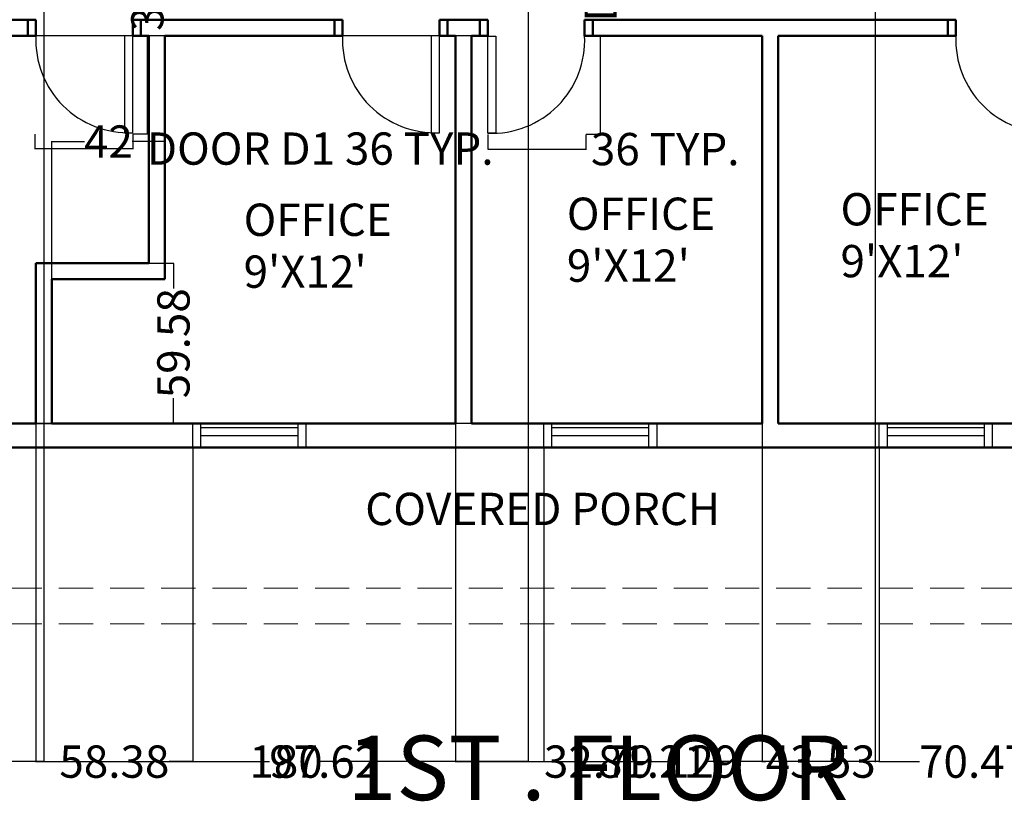
# Model space of a CAD drawing. Units: inches. Extents: x 128 to 1267, y -109 to 1208.
# Tile 2 of 8: x 418 to 784, y -97 to 194. Entities that reach past the tile are written whole.
import ezdxf

# ---------------------------------------------------------------- set-up
doc = ezdxf.new("R2010")
doc.units = ezdxf.units.IN
doc.header["$MEASUREMENT"] = 0
doc.linetypes.add('DASHED', pattern=[19.05, 12.7, -6.35])
for name, color, linetype, lineweight in [('A-ANNO-DIMS', 2, 'Continuous', 18), ('A-ANNO-TEXT', 7, 'Continuous', 35), ('A-AREA-IDEN', 3, 'Continuous', 25), ('A-DOOR', 4, 'Continuous', 25), ('A-GLAZ', 3, 'Continuous', 25), ('A-ROOF-OVHD', 9, 'DASHED', 18), ('A-WALL', 7, 'Continuous', 50)]:
    doc.layers.add(name, color=color, linetype=linetype, lineweight=lineweight)
doc.styles.get("Standard").update_dxf_attribs({"font": 'arial.ttf'})
doc.dimstyles.get("Standard").update_dxf_attribs({"dimtxt": 12, "dimasz": 0.18, "dimexe": 0.18, "dimexo": 0.0625, "dimgap": 0.09, "dimtad": 0, "dimdec": 1, "dimzin": 0, "dimdsep": 46, "dimlunit": 3, "dimtxsty": 'Standard', "dimcen": 0.09, "dimadec": 0, "dimazin": 0, "dimtfac": 1, "dimtdec": 1, "dimtofl": 0, "dimtmove": 0, "dimatfit": 3, "dimfxl": 1, "dimtolj": 1, "dimtzin": 0, "dimarcsym": 0})

# ---------------------------------------------------------------- blocks, each defined once
blk = doc.blocks.new('DOOR-900')
blk.add_lwpolyline([(460.06, 187.64), (457.06, 187.64), (457.06, 151.64), (460.06, 151.64)], close=True)
blk.add_arc((458.56, 186.14), 34.53, 177.5104, 272.4896)
blk = doc.blocks.new('DOOR-875')
blk.add_lwpolyline([(592.06, 187.47), (595.06, 187.47), (595.06, 151.47), (592.06, 151.47)], close=True)
blk.add_arc((593.56, 185.98), 34.54, 267.511, 2.7608)
blk = doc.blocks.new('WIN-900')
for p, q in [((1102.06, 345.56), (1111.06, 345.56)), ((1102.06, 342.56), (1111.06, 342.56)), ((1103.56, 306.56), (1103.56, 342.56)), ((1106.56, 306.56), (1106.56, 342.56)), ((1111.06, 306.56), (1102.06, 306.56)), ((1111.06, 303.56), (1102.06, 303.56))]:
    blk.add_line(p, q)
blk = doc.blocks.new('*D10')
at = {"layer": 'A-ANNO-DIMS', "color": 0, "lineweight": -2, "transparency": 16777216}
for p, q in [((423.64, 151.16), (423.64, 145.58)), ((460.06, 151.16), (460.06, 145.58)), ((423.82, 145.76), (459.88, 145.76)), ((460.06, 145.76), (460.24, 145.76))]:
    blk.add_line(p, q, dxfattribs=at)
at = {"layer": 'A-ANNO-DIMS', "color": 0, "transparency": 16777216}
for points in [[(423.82, 145.79), (423.82, 145.73), (423.64, 145.76)], [(459.88, 145.79), (459.88, 145.73), (460.06, 145.76)]]:
    blk.add_solid(points, dxfattribs=at)
at = {"layer": 'Defpoints', "color": 0, "transparency": 16777216}
for p in [(423.64, 151.22), (460.06, 151.22), (460.06, 145.76)]:
    blk.add_point(p, dxfattribs=at)
at = {"layer": 'A-ANNO-DIMS', "color": 0, "transparency": 16777216, "insert": (529.75, 145.76), "char_height": 12, "attachment_point": 5}
blk.add_mtext('\\A1;DOOR D1 36 TYP.', dxfattribs=at)
blk = doc.blocks.new('*D11')
at = {"layer": 'A-ANNO-DIMS', "color": 0, "lineweight": -2, "transparency": 16777216}
for p, q in [((460.12, 187.64), (465.7, 187.64)), ((465.52, 187.64), (465.52, 187.82)), ((465.52, 151.4), (465.52, 187.46)), ((460.12, 151.22), (465.7, 151.22))]:
    blk.add_line(p, q, dxfattribs=at)
at = {"layer": 'A-ANNO-DIMS', "color": 0, "transparency": 16777216}
for points in [[(465.49, 187.46), (465.55, 187.46), (465.52, 187.64)], [(465.49, 151.4), (465.55, 151.4), (465.52, 151.22)]]:
    blk.add_solid(points, dxfattribs=at)
at = {"layer": 'Defpoints', "color": 0, "transparency": 16777216}
for p in [(460.06, 187.64), (465.52, 187.64), (460.06, 151.22)]:
    blk.add_point(p, dxfattribs=at)
at = {"layer": 'A-ANNO-DIMS', "color": 0, "transparency": 16777216, "insert": (465.52, 217.11), "char_height": 12, "attachment_point": 5, "rotation": 90}
blk.add_mtext('\\A1;36 TYP.', dxfattribs=at)
blk = doc.blocks.new('*D20')
at = {"layer": 'A-ANNO-DIMS', "color": 0, "lineweight": -2, "transparency": 16777216}
for p, q in [((628.59, 187.64), (634.19, 187.64)), ((634.01, 187.64), (634.01, 187.82)), ((634.01, 151.23), (634.01, 187.46)), ((628.59, 151.05), (634.19, 151.05))]:
    blk.add_line(p, q, dxfattribs=at)
at = {"layer": 'A-ANNO-DIMS', "color": 0, "transparency": 16777216}
for points in [[(633.98, 187.46), (634.04, 187.46), (634.01, 187.64)], [(633.98, 151.23), (634.04, 151.23), (634.01, 151.05)]]:
    blk.add_solid(points, dxfattribs=at)
at = {"layer": 'Defpoints', "color": 0, "transparency": 16777216}
for p in [(628.52, 187.64), (634.01, 187.64), (628.52, 151.05)]:
    blk.add_point(p, dxfattribs=at)
at = {"layer": 'A-ANNO-DIMS', "color": 0, "transparency": 16777216, "insert": (634.01, 257.34), "char_height": 12, "attachment_point": 5, "rotation": 90}
blk.add_mtext('\\A1;DOOR D2 37 TYP.', dxfattribs=at)
blk = doc.blocks.new('*D21')
at = {"layer": 'A-ANNO-DIMS', "color": 0, "lineweight": -2, "transparency": 16777216}
for p, q in [((592.06, 150.98), (592.06, 145.38)), ((628.52, 150.98), (628.52, 145.38)), ((592.24, 145.56), (628.34, 145.56)), ((628.52, 145.56), (628.7, 145.56))]:
    blk.add_line(p, q, dxfattribs=at)
at = {"layer": 'A-ANNO-DIMS', "color": 0, "transparency": 16777216}
for points in [[(592.24, 145.59), (592.24, 145.53), (592.06, 145.56)], [(628.34, 145.59), (628.34, 145.53), (628.52, 145.56)]]:
    blk.add_solid(points, dxfattribs=at)
at = {"layer": 'Defpoints', "color": 0, "transparency": 16777216}
for p in [(592.06, 151.05), (628.52, 151.05), (628.52, 145.56)]:
    blk.add_point(p, dxfattribs=at)
at = {"layer": 'A-ANNO-DIMS', "color": 0, "transparency": 16777216, "insert": (658, 145.56), "char_height": 12, "attachment_point": 5}
blk.add_mtext('\\A1;36 TYP.', dxfattribs=at)
blk = doc.blocks.new('*D22')
at = {"layer": 'A-ANNO-DIMS', "color": 0, "lineweight": -2, "transparency": 16777216}
for p, q in [((223.06, -17.52), (223.06, 495.44)), ((223.24, 495.26), (653.69, 495.26)), ((1110.88, 495.26), (680.42, 495.26)), ((1111.06, -17.52), (1111.06, 495.44))]:
    blk.add_line(p, q, dxfattribs=at)
at = {"layer": 'A-ANNO-DIMS', "color": 0, "transparency": 16777216}
for points in [[(223.24, 495.29), (223.24, 495.23), (223.06, 495.26)], [(1110.88, 495.29), (1110.88, 495.23), (1111.06, 495.26)]]:
    blk.add_solid(points, dxfattribs=at)
at = {"layer": 'Defpoints', "color": 0, "transparency": 16777216}
for p in [(1111.06, 495.26), (223.06, -17.58), (1111.06, -17.58)]:
    blk.add_point(p, dxfattribs=at)
at = {"layer": 'A-ANNO-DIMS', "color": 0, "transparency": 16777216, "insert": (667.06, 495.26), "char_height": 12, "attachment_point": 5}
blk.add_mtext('\\A1;888', dxfattribs=at)
blk = doc.blocks.new('*D29')
at = {"layer": 'A-ANNO-DIMS', "color": 0, "lineweight": -2, "transparency": 16777216}
for p, q in [((424.06, 43.58), (424.06, -82.19)), ((304.35, 34.58), (304.35, -82.19)), ((304.53, -82.01), (344.43, -82.01)), ((423.88, -82.01), (383.97, -82.01))]:
    blk.add_line(p, q, dxfattribs=at)
at = {"layer": 'A-ANNO-DIMS', "color": 0, "transparency": 16777216}
for points in [[(304.53, -81.98), (304.53, -82.04), (304.35, -82.01)], [(423.88, -81.98), (423.88, -82.04), (424.06, -82.01)]]:
    blk.add_solid(points, dxfattribs=at)
at = {"layer": 'Defpoints', "color": 0, "transparency": 16777216}
for p in [(424.06, 43.64), (304.35, 34.64), (424.06, -82.01)]:
    blk.add_point(p, dxfattribs=at)
at = {"layer": 'A-ANNO-DIMS', "color": 0, "transparency": 16777216, "insert": (364.2, -82.01), "char_height": 12, "attachment_point": 5}
blk.add_mtext('\\A1;119.7', dxfattribs=at)
blk = doc.blocks.new('*D30')
at = {"layer": 'A-ANNO-DIMS', "color": 0, "lineweight": -2, "transparency": 16777216}
for p, q in [((424.06, 43.58), (424.06, -82.19)), ((482.44, 34.58), (482.44, -82.19)), ((424.24, -82.01), (432.9, -82.01)), ((482.26, -82.01), (473.6, -82.01))]:
    blk.add_line(p, q, dxfattribs=at)
at = {"layer": 'A-ANNO-DIMS', "color": 0, "transparency": 16777216}
for points in [[(424.24, -81.98), (424.24, -82.04), (424.06, -82.01)], [(482.26, -81.98), (482.26, -82.04), (482.44, -82.01)]]:
    blk.add_solid(points, dxfattribs=at)
at = {"layer": 'Defpoints', "color": 0, "transparency": 16777216}
for p in [(424.06, 43.64), (482.44, 34.64), (482.44, -82.01)]:
    blk.add_point(p, dxfattribs=at)
at = {"layer": 'A-ANNO-DIMS', "color": 0, "transparency": 16777216, "insert": (453.25, -82.01), "char_height": 12, "attachment_point": 5}
blk.add_mtext('\\A1;58.38', dxfattribs=at)
blk = doc.blocks.new('*D31')
at = {"layer": 'A-ANNO-DIMS', "color": 0, "lineweight": -2, "transparency": 16777216}
for p, q in [((580.06, 43.58), (580.06, -82.19)), ((482.44, 34.58), (482.44, -82.19)), ((482.62, -82.01), (510.97, -82.01)), ((579.88, -82.01), (551.52, -82.01))]:
    blk.add_line(p, q, dxfattribs=at)
at = {"layer": 'A-ANNO-DIMS', "color": 0, "transparency": 16777216}
for points in [[(482.62, -81.98), (482.62, -82.04), (482.44, -82.01)], [(579.88, -81.98), (579.88, -82.04), (580.06, -82.01)]]:
    blk.add_solid(points, dxfattribs=at)
at = {"layer": 'Defpoints', "color": 0, "transparency": 16777216}
for p in [(580.06, 43.64), (482.44, 34.64), (580.06, -82.01)]:
    blk.add_point(p, dxfattribs=at)
at = {"layer": 'A-ANNO-DIMS', "color": 0, "transparency": 16777216, "insert": (531.25, -82.01), "char_height": 12, "attachment_point": 5}
blk.add_mtext('\\A1;97.62', dxfattribs=at)
blk = doc.blocks.new('*D32')
at = {"layer": 'A-ANNO-DIMS', "color": 0, "lineweight": -2, "transparency": 16777216}
for p, q in [((580.06, 43.58), (580.06, -82.19)), ((612.84, 34.58), (612.84, -82.19)), ((580.24, -82.01), (612.66, -82.01)), ((612.84, -82.01), (613.02, -82.01))]:
    blk.add_line(p, q, dxfattribs=at)
at = {"layer": 'A-ANNO-DIMS', "color": 0, "transparency": 16777216}
for points in [[(580.24, -81.98), (580.24, -82.04), (580.06, -82.01)], [(612.66, -81.98), (612.66, -82.04), (612.84, -82.01)]]:
    blk.add_solid(points, dxfattribs=at)
at = {"layer": 'Defpoints', "color": 0, "transparency": 16777216}
for p in [(580.06, 43.64), (612.84, 34.64), (612.84, -82.01)]:
    blk.add_point(p, dxfattribs=at)
at = {"layer": 'A-ANNO-DIMS', "color": 0, "transparency": 16777216, "insert": (633.37, -82.01), "char_height": 12, "attachment_point": 5}
blk.add_mtext('\\A1;32.79', dxfattribs=at)
blk = doc.blocks.new('*D33')
at = {"layer": 'A-ANNO-DIMS', "color": 0, "lineweight": -2, "transparency": 16777216}
for p, q in [((694.06, 43.58), (694.06, -82.19)), ((612.84, 34.58), (612.84, -82.19)), ((613.02, -82.01), (634.26, -82.01)), ((693.88, -82.01), (672.64, -82.01))]:
    blk.add_line(p, q, dxfattribs=at)
at = {"layer": 'A-ANNO-DIMS', "color": 0, "transparency": 16777216}
for points in [[(613.02, -81.98), (613.02, -82.04), (612.84, -82.01)], [(693.88, -81.98), (693.88, -82.04), (694.06, -82.01)]]:
    blk.add_solid(points, dxfattribs=at)
at = {"layer": 'Defpoints', "color": 0, "transparency": 16777216}
for p in [(694.06, 43.64), (612.84, 34.64), (694.06, -82.01)]:
    blk.add_point(p, dxfattribs=at)
at = {"layer": 'A-ANNO-DIMS', "color": 0, "transparency": 16777216, "insert": (653.45, -82.01), "char_height": 12, "attachment_point": 5}
blk.add_mtext('\\A1;81.21', dxfattribs=at)
blk = doc.blocks.new('*D34')
at = {"layer": 'A-ANNO-DIMS', "color": 0, "lineweight": -2, "transparency": 16777216}
for p, q in [((694.06, 43.58), (694.06, -82.19)), ((737.59, 34.58), (737.59, -82.19)), ((694.24, -82.01), (695.24, -82.01)), ((737.41, -82.01), (736.4, -82.01))]:
    blk.add_line(p, q, dxfattribs=at)
at = {"layer": 'A-ANNO-DIMS', "color": 0, "transparency": 16777216}
for points in [[(694.24, -81.98), (694.24, -82.04), (694.06, -82.01)], [(737.41, -81.98), (737.41, -82.04), (737.59, -82.01)]]:
    blk.add_solid(points, dxfattribs=at)
at = {"layer": 'Defpoints', "color": 0, "transparency": 16777216}
for p in [(694.06, 43.64), (737.59, 34.64), (737.59, -82.01)]:
    blk.add_point(p, dxfattribs=at)
at = {"layer": 'A-ANNO-DIMS', "color": 0, "transparency": 16777216, "insert": (715.82, -82.01), "char_height": 12, "attachment_point": 5}
blk.add_mtext('\\A1;43.53', dxfattribs=at)
blk = doc.blocks.new('*D35')
at = {"layer": 'A-ANNO-DIMS', "color": 0, "lineweight": -2, "transparency": 16777216}
for p, q in [((808.06, 43.58), (808.06, -82.19)), ((737.59, 34.58), (737.59, -82.19)), ((737.77, -82.01), (752.54, -82.01)), ((807.88, -82.01), (793.11, -82.01))]:
    blk.add_line(p, q, dxfattribs=at)
at = {"layer": 'A-ANNO-DIMS', "color": 0, "transparency": 16777216}
for points in [[(737.77, -81.98), (737.77, -82.04), (737.59, -82.01)], [(807.88, -81.98), (807.88, -82.04), (808.06, -82.01)]]:
    blk.add_solid(points, dxfattribs=at)
at = {"layer": 'Defpoints', "color": 0, "transparency": 16777216}
for p in [(808.06, 43.64), (737.59, 34.64), (808.06, -82.01)]:
    blk.add_point(p, dxfattribs=at)
at = {"layer": 'A-ANNO-DIMS', "color": 0, "transparency": 16777216, "insert": (772.82, -82.01), "char_height": 12, "attachment_point": 5}
blk.add_mtext('\\A1;70.47', dxfattribs=at)
blk = doc.blocks.new('*D76')
at = {"layer": 'A-ANNO-DIMS', "color": 0, "lineweight": -2, "transparency": 16777216}
for p, q in [((373.06, 295.58), (373.06, -82.19)), ((427.06, 295.58), (427.06, -82.19)), ((373.24, -82.01), (391.4, -82.01)), ((426.88, -82.01), (408.72, -82.01))]:
    blk.add_line(p, q, dxfattribs=at)
at = {"layer": 'A-ANNO-DIMS', "color": 0, "transparency": 16777216}
for points in [[(373.24, -81.98), (373.24, -82.04), (373.06, -82.01)], [(426.88, -81.98), (426.88, -82.04), (427.06, -82.01)]]:
    blk.add_solid(points, dxfattribs=at)
at = {"layer": 'Defpoints', "color": 0, "transparency": 16777216}
for p in [(373.06, 295.64), (427.06, 295.64), (427.06, -82.01)]:
    blk.add_point(p, dxfattribs=at)
at = {"layer": 'A-ANNO-DIMS', "color": 0, "transparency": 16777216, "insert": (400.06, -82.01), "char_height": 12, "attachment_point": 5}
blk.add_mtext('\\A1;54', dxfattribs=at)
blk = doc.blocks.new('*D77')
at = {"layer": 'A-ANNO-DIMS', "color": 0, "lineweight": -2, "transparency": 16777216}
for p, q in [((427.06, 295.58), (427.06, -82.19)), ((607.06, 295.58), (607.06, -82.19)), ((427.24, -82.01), (504.29, -82.01)), ((606.88, -82.01), (529.82, -82.01))]:
    blk.add_line(p, q, dxfattribs=at)
at = {"layer": 'A-ANNO-DIMS', "color": 0, "transparency": 16777216}
for points in [[(427.24, -81.98), (427.24, -82.04), (427.06, -82.01)], [(606.88, -81.98), (606.88, -82.04), (607.06, -82.01)]]:
    blk.add_solid(points, dxfattribs=at)
at = {"layer": 'Defpoints', "color": 0, "transparency": 16777216}
for p in [(427.06, 295.64), (607.06, 295.64), (607.06, -82.01)]:
    blk.add_point(p, dxfattribs=at)
at = {"layer": 'A-ANNO-DIMS', "color": 0, "transparency": 16777216, "insert": (517.06, -82.01), "char_height": 12, "attachment_point": 5}
blk.add_mtext('\\A1;180', dxfattribs=at)
blk = doc.blocks.new('*D78')
at = {"layer": 'A-ANNO-DIMS', "color": 0, "lineweight": -2, "transparency": 16777216}
for p, q in [((607.06, 295.58), (607.06, -82.19)), ((736.06, 295.58), (736.06, -82.19)), ((607.24, -82.01), (658.76, -82.01)), ((735.88, -82.01), (684.35, -82.01))]:
    blk.add_line(p, q, dxfattribs=at)
at = {"layer": 'A-ANNO-DIMS', "color": 0, "transparency": 16777216}
for points in [[(607.24, -81.98), (607.24, -82.04), (607.06, -82.01)], [(735.88, -81.98), (735.88, -82.04), (736.06, -82.01)]]:
    blk.add_solid(points, dxfattribs=at)
at = {"layer": 'Defpoints', "color": 0, "transparency": 16777216}
for p in [(607.06, 295.64), (736.06, 295.64), (736.06, -82.01)]:
    blk.add_point(p, dxfattribs=at)
at = {"layer": 'A-ANNO-DIMS', "color": 0, "transparency": 16777216, "insert": (671.56, -82.01), "char_height": 12, "attachment_point": 5}
blk.add_mtext('\\A1;129', dxfattribs=at)
blk = doc.blocks.new('*D85')
at = {"layer": 'A-ANNO-DIMS', "color": 0, "lineweight": -2, "transparency": 16777216}
for p, q in [((585.99, 187.64), (135.73, 187.64)), ((135.91, 187.46), (135.91, 128.4)), ((135.91, 43.82), (135.91, 102.88)), ((585.99, 43.64), (135.73, 43.64))]:
    blk.add_line(p, q, dxfattribs=at)
at = {"layer": 'A-ANNO-DIMS', "color": 0, "transparency": 16777216}
for points in [[(135.88, 187.46), (135.94, 187.46), (135.91, 187.64)], [(135.88, 43.82), (135.94, 43.82), (135.91, 43.64)]]:
    blk.add_solid(points, dxfattribs=at)
at = {"layer": 'Defpoints', "color": 0, "transparency": 16777216}
for p in [(586.06, 187.64), (135.91, 43.64), (586.06, 43.64)]:
    blk.add_point(p, dxfattribs=at)
at = {"layer": 'A-ANNO-DIMS', "color": 0, "transparency": 16777216, "insert": (135.91, 115.64), "char_height": 12, "attachment_point": 5, "rotation": 90}
blk.add_mtext('\\A1;144', dxfattribs=at)
blk = doc.blocks.new('*D86')
at = {"layer": 'A-ANNO-DIMS', "color": 0, "lineweight": -2, "transparency": 16777216}
for p, q in [((424.12, 103.22), (475.39, 103.22)), ((475.21, 103.04), (475.21, 93.78)), ((475.21, 43.82), (475.21, 53.08)), ((424.12, 43.64), (475.39, 43.64))]:
    blk.add_line(p, q, dxfattribs=at)
at = {"layer": 'A-ANNO-DIMS', "color": 0, "transparency": 16777216}
for points in [[(475.18, 103.04), (475.24, 103.04), (475.21, 103.22)], [(475.18, 43.82), (475.24, 43.82), (475.21, 43.64)]]:
    blk.add_solid(points, dxfattribs=at)
at = {"layer": 'Defpoints', "color": 0, "transparency": 16777216}
for p in [(424.06, 103.22), (424.06, 43.64), (475.21, 43.64)]:
    blk.add_point(p, dxfattribs=at)
at = {"layer": 'A-ANNO-DIMS', "color": 0, "transparency": 16777216, "insert": (475.21, 73.43), "char_height": 12, "attachment_point": 5, "rotation": 90}
blk.add_mtext('\\A1;59.58', dxfattribs=at)
blk = doc.blocks.new('*D87')
at = {"layer": 'A-ANNO-DIMS', "color": 0, "lineweight": -2, "transparency": 16777216}
for p, q in [((430.06, 97.28), (430.06, 148.55)), ((430.24, 148.37), (442.19, 148.37)), ((471.88, 148.37), (459.92, 148.37)), ((472.06, 97.28), (472.06, 148.55))]:
    blk.add_line(p, q, dxfattribs=at)
at = {"layer": 'A-ANNO-DIMS', "color": 0, "transparency": 16777216}
for points in [[(430.24, 148.4), (430.24, 148.34), (430.06, 148.37)], [(471.88, 148.4), (471.88, 148.34), (472.06, 148.37)]]:
    blk.add_solid(points, dxfattribs=at)
at = {"layer": 'Defpoints', "color": 0, "transparency": 16777216}
for p in [(472.06, 148.37), (430.06, 97.22), (472.06, 97.22)]:
    blk.add_point(p, dxfattribs=at)
at = {"layer": 'A-ANNO-DIMS', "color": 0, "transparency": 16777216, "insert": (451.06, 148.37), "char_height": 12, "attachment_point": 5}
blk.add_mtext('\\A1;42', dxfattribs=at)

msp = doc.modelspace()

# ---------------------------------------------------------------- linework, layer by layer
at = {"layer": 'A-ROOF-OVHD'}
for p, q in [((223.056, -17.5809), (1111.056, -17.5809)), ((223.056, -30.8598), (1111.056, -30.8598))]:
    msp.add_line(p, q, dxfattribs=at)
at = {"layer": 'A-WALL'}
for p, q in [((313.056, 193.6399), (424.056, 193.6399)), ((421.056, 187.6399), (421.056, 193.6399)), ((424.056, 187.6399), (424.056, 193.6399)), ((460.056, 187.6399), (460.056, 193.6399)), ((460.056, 193.6399), (538.056, 193.6399)), ((463.056, 187.6399), (463.056, 193.6399)), ((535.056, 187.6399), (535.056, 193.6399)), ((538.056, 187.6399), (538.056, 193.6399)), ((574.056, 187.6399), (574.056, 193.6399)), ((574.056, 193.6399), (592.056, 193.6399)), ((577.056, 187.6399), (577.056, 193.6399)), ((589.056, 187.6399), (589.056, 193.6399)), ((592.056, 187.6399), (592.056, 193.6399)), ((628.056, 187.6399), (628.056, 193.6399)), ((628.056, 193.6399), (766.056, 193.6399)), ((631.056, 187.6399), (631.056, 193.6399)), ((763.056, 187.6399), (763.056, 193.6399)), ((766.056, 187.6399), (766.056, 193.6399)), ((282.6423, 187.6399), (424.056, 187.6399)), ((460.056, 187.6399), (466.056, 187.6399)), ((466.056, 187.6399), (466.056, 103.2163)), ((472.056, 187.6399), (472.056, 97.2163)), ((472.056, 187.6399), (538.056, 187.6399)), ((574.056, 187.6399), (580.056, 187.6399)), ((580.056, 187.6399), (580.056, 43.6399)), ((586.056, 187.6399), (586.056, 43.6399)), ((586.056, 187.6399), (592.056, 187.6399)), ((628.056, 187.6399), (694.056, 187.6399)), ((694.056, 187.6399), (694.056, 43.6399)), ((700.056, 187.6399), (700.056, 43.6399)), ((700.056, 187.6399), (766.056, 187.6399)), ((424.056, 103.2163), (424.056, 43.6399)), ((424.056, 103.2163), (466.056, 103.2163)), ((430.056, 97.2163), (430.056, 43.6399)), ((430.056, 97.2163), (472.056, 97.2163)), ((232.056, 43.6399), (424.056, 43.6399)), ((430.056, 43.6399), (580.056, 43.6399)), ((586.056, 43.6399), (694.056, 43.6399)), ((700.056, 43.6399), (808.056, 43.6399))]:
    msp.add_line(p, q, dxfattribs=at)
msp.add_lwpolyline([(223.056, 199.6399), (223.056, 34.6399), (1024.056, 34.6399)], dxfattribs=at)

# ---------------------------------------------------------------- block references
at = {"layer": 'A-DOOR'}
for name, p in [('DOOR-900', (0, 0)), ('DOOR-900', (114, 0)), ('DOOR-875', (0, 0)), ('DOOR-900', (342, 0))]:
    msp.add_blockref(name, p, dxfattribs=at)
at = {"layer": 'A-GLAZ', "rotation": 270.0000000000005}
for p in [(178.8764, 1145.696), (309.281, 1145.696), (434.0277, 1145.696)]:
    msp.add_blockref('WIN-900', p, dxfattribs=at)

# ---------------------------------------------------------------- texts
at = {"layer": 'A-ANNO-TEXT'}
msp.add_text('1ST . FLOOR', height=24, dxfattribs=at).set_placement((539.8514, -96.3292))
at = {"layer": 'A-AREA-IDEN'}
for s, p in [('OFFICE', (723.1619, 117.2145)), ('OFFICE', (501.2887, 113.3056)), ('OFFICE', (621.4467, 115.5393)), ("9'X12'", (723.1619, 97.9376)), ("9'X12'", (501.2887, 94.0287)), ("9'X12'", (621.4467, 96.2624)), ('COVERED PORCH', (546.4945, 5.8718))]:
    msp.add_text(s, height=12, dxfattribs=at).set_placement(p)

# ---------------------------------------------------------------- dimensions: what is measured, and where the dimension line sits
at = {"layer": 'A-ANNO-DIMS'}
for base, p1, p2, override, picture, middle in [((1111.056, 495.2611), (223.056, -17.5809), (1111.056, -17.5809), {"dimdec": 0, "dimlfac": 1, "dimrnd": 0, "dimzin": 0, "dimdsep": 46, "dimlunit": 2}, '*D22', (667.056, 495.2611)), ((427.056, -82.0098), (373.056, 295.6399), (427.056, 295.6399), {"dimdec": 0, "dimlfac": 1, "dimrnd": 0, "dimzin": 0, "dimdsep": 46, "dimlunit": 2}, '*D76', (400.056, -82.0098)), ((607.056, -82.0098), (427.056, 295.6399), (607.056, 295.6399), {"dimdec": 0, "dimlfac": 1, "dimrnd": 0, "dimzin": 0, "dimdsep": 46, "dimlunit": 2}, '*D77', (517.056, -82.0098)), ((736.056, -82.0098), (607.056, 295.6399), (736.056, 295.6399), {"dimdec": 0, "dimlfac": 1, "dimrnd": 0, "dimzin": 0, "dimdsep": 46, "dimlunit": 2}, '*D78', (671.556, -82.0098)), ((472.056, 148.3663), (430.056, 97.2163), (472.056, 97.2163), {"dimdec": 0, "dimlfac": 1, "dimrnd": 0, "dimzin": 0, "dimdsep": 46, "dimlunit": 2}, '*D87', (451.056, 148.3663)), ((424.056, -82.0098), (304.3472, 34.6399), (424.056, 43.6399), {"dimdec": 1, "dimlfac": 1, "dimrnd": 0, "dimzin": 0, "dimdsep": 46, "dimlunit": 2}, '*D29', (364.2016, -82.0098)), ((482.4387, -82.0098), (424.056, 43.6399), (482.4387, 34.6399), {"dimdec": 2, "dimlfac": 1, "dimrnd": 0, "dimzin": 0, "dimdsep": 46, "dimlunit": 2}, '*D30', (453.2474, -82.0098)), ((580.056, -82.0098), (482.4387, 34.6399), (580.056, 43.6399), {"dimdec": 2, "dimlfac": 1, "dimrnd": 0, "dimzin": 0, "dimdsep": 46, "dimlunit": 2}, '*D31', (531.2474, -82.0098)), ((612.8433, -82.0098), (580.056, 43.6399), (612.8433, 34.6399), {"dimdec": 2, "dimlfac": 1, "dimrnd": 0, "dimzin": 0, "dimdsep": 46, "dimlunit": 2}, '*D32', (633.3684, -82.0098)), ((694.056, -82.0098), (612.8433, 34.6399), (694.056, 43.6399), {"dimdec": 2, "dimlfac": 1, "dimrnd": 0, "dimzin": 0, "dimdsep": 46, "dimlunit": 2}, '*D33', (653.4497, -82.0098)), ((737.59, -82.0098), (694.056, 43.6399), (737.59, 34.6399), {"dimdec": 2, "dimlfac": 1, "dimrnd": 0, "dimzin": 0, "dimdsep": 46, "dimlunit": 2}, '*D34', (715.823, -82.0098)), ((808.056, -82.0098), (737.59, 34.6399), (808.056, 43.6399), {"dimdec": 2, "dimlfac": 1, "dimrnd": 0, "dimzin": 0, "dimdsep": 46, "dimlunit": 2}, '*D35', (772.823, -82.0098))]:
    dim = msp.add_linear_dim(base=base, p1=p1, p2=p2, dimstyle='Standard', override=override, dxfattribs=at)
    dim.commit()
    dim.dimension.update_dxf_attribs({"geometry": picture, "text_midpoint": middle})
for base, p1, p2, text, picture, middle in [((634.0127, 187.6399), (628.5237, 151.0471), (628.5237, 187.6399), 'DOOR D2 <> TYP.', '*D20', (634.0127, 257.3356)), ((465.5191, 187.6399), (460.056, 151.2195), (460.056, 187.6399), '<> TYP.', '*D11', (465.5191, 217.1118))]:
    dim = msp.add_linear_dim(base=base, p1=p1, p2=p2, angle=90, text=text, dimstyle='Standard', override={"dimdec": 0, "dimrnd": 0, "dimzin": 0, "dimlunit": 2}, dxfattribs=at)
    dim.commit()
    dim.dimension.update_dxf_attribs({"geometry": picture, "text_midpoint": middle})
for base, p1, p2, angle, override, picture, middle in [((135.906, 43.6399), (586.056, 187.6399), (586.056, 43.6399), 90, {"dimdec": 0, "dimlfac": 1, "dimrnd": 0, "dimzin": 0, "dimdsep": 46, "dimlunit": 2}, '*D85', (135.906, 115.6399)), ((475.206, 43.6399), (424.056, 103.2163), (424.056, 43.6399), 270, {"dimdec": 2, "dimlfac": 1, "dimrnd": 0, "dimzin": 0, "dimdsep": 46, "dimlunit": 2}, '*D86', (475.206, 73.4281))]:
    dim = msp.add_linear_dim(base=base, p1=p1, p2=p2, angle=angle, dimstyle='Standard', override=override, dxfattribs=at)
    dim.commit()
    dim.dimension.update_dxf_attribs({"geometry": picture, "text_midpoint": middle})
for base, p1, p2, text, picture, middle in [((460.056, 145.7564), (423.6356, 151.2195), (460.056, 151.2195), 'DOOR D1 <> TYP.', '*D10', (529.7517, 145.7564)), ((628.5237, 145.5581), (592.056, 151.0471), (628.5237, 151.0471), '<> TYP.', '*D21', (657.9956, 145.5581))]:
    dim = msp.add_linear_dim(base=base, p1=p1, p2=p2, text=text, dimstyle='Standard', override={"dimdec": 0, "dimrnd": 0, "dimzin": 0, "dimlunit": 2}, dxfattribs=at)
    dim.commit()
    dim.dimension.update_dxf_attribs({"geometry": picture, "text_midpoint": middle})

doc.saveas('drawing.dxf')
